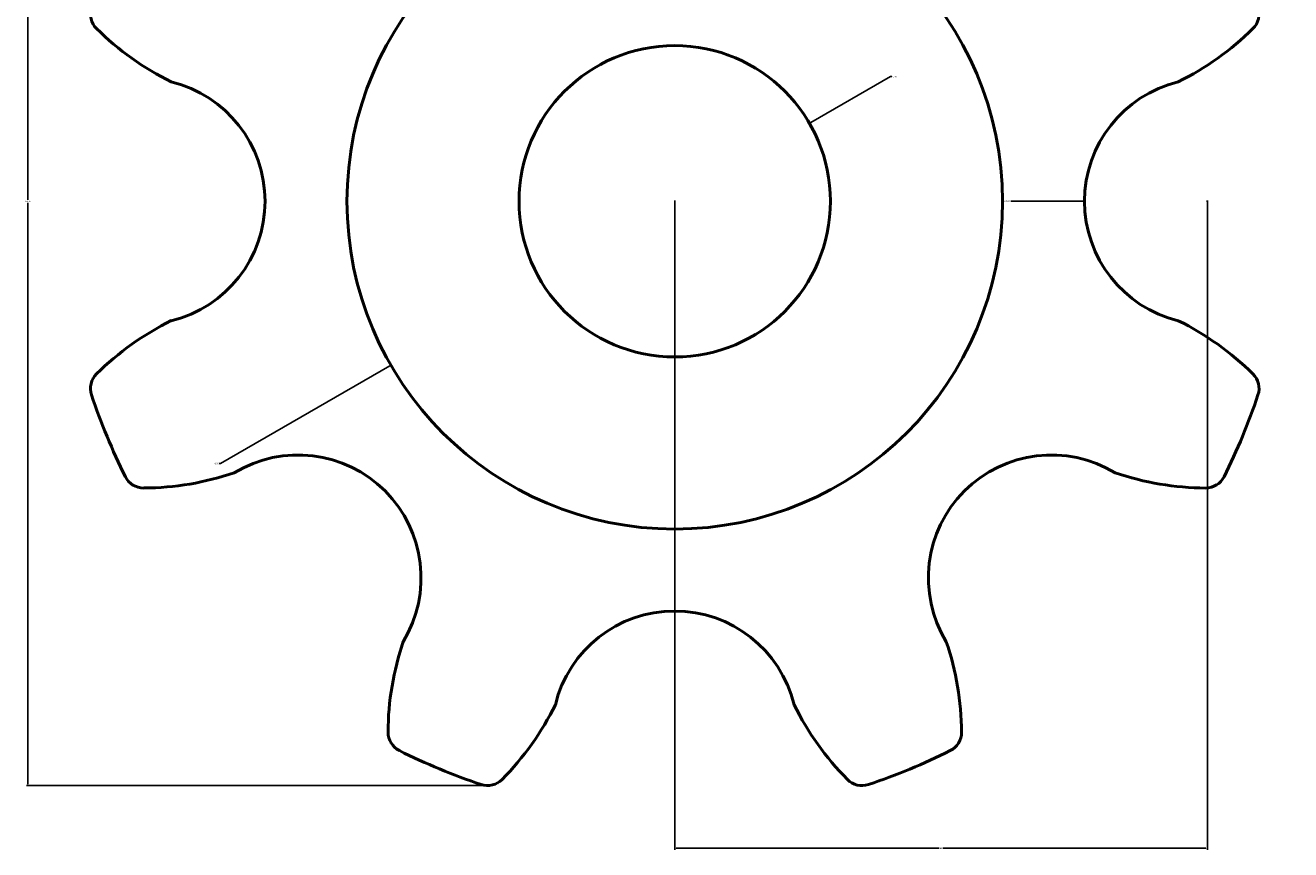
# Model space of a CAD drawing. Units: millimetres. Extents: x 7298 to 7452, y 8725 to 8883.
# Tile 1 of 2: x 7298 to 7452, y 8725 to 8826. Entities that reach past the tile are written whole.
import ezdxf

# ---------------------------------------------------------------- set-up
doc = ezdxf.new("R2010")
doc.units = ezdxf.units.MM
doc.layers.add('M-DIMS', color=2, linetype='Continuous', lineweight=18)
doc.layers.add('M-OUTL', color=7, linetype='Continuous', lineweight=50)
doc.styles.get("Standard").update_dxf_attribs({"font": 'arial.ttf'})
doc.dimstyles.get("Standard").update_dxf_attribs({"dimtxt": 0.18, "dimasz": 0.18, "dimexe": 0.18, "dimexo": 0.0625, "dimgap": 0.09, "dimtad": 0, "dimtih": 1, "dimtoh": 1, "dimdec": 4, "dimzin": 0, "dimdsep": 46, "dimtxsty": 'Standard', "dimcen": 0.09, "dimadec": 0, "dimazin": 0, "dimtfac": 1, "dimtdec": 4, "dimtofl": 0, "dimtmove": 0, "dimatfit": 3, "dimfxl": 1, "dimtolj": 1, "dimtzin": 0, "dimarcsym": 0})

# ---------------------------------------------------------------- blocks, each defined once
blk = doc.blocks.new('*U1')
for centre, radius, start, end in [((-2.28, 7.71), 2.5, 89.661, 153.3674), ((-2.47, -24.79), 35, 71.2539, 89.661), ((62.53, -24.79), 75, 153.3674, 161.6326), ((-6.28, -1.94), 2.5, 161.6326, 225.339), ((16.57, 21.18), 35, 225.339, 243.7461)]:
    blk.add_arc(centre, radius, start, end)
blk = doc.blocks.new('*U2')
at = {"layer": 'M-OUTL', "color": 0, "linetype": 'ByBlock', "lineweight": -2, "transparency": 16777216}
for p, rotation in [((7350.2, 8866.09), 315.0000000000001), ((7401.68, 8866.87), 270), ((7438.63, 8831.03), 225), ((7315.15, 8777.66), 44.99999999999996), ((7439.42, 8779.56), 180), ((7403.58, 8742.6), 134.9999999999999), ((7352.11, 8741.82), 90)]:
    blk.add_blockref('*U1', p, dxfattribs=dict(at, rotation=rotation))
blk.add_blockref('*U1', (7314.36, 8829.13), dxfattribs=at)
blk = doc.blocks.new('*D4')
at = {"layer": 'Defpoints', "color": 0, "transparency": 16777216}
for p in [(7297.94, 8875.65), (7353.95, 8875.65), (7353.95, 8733.04)]:
    blk.add_point(p, dxfattribs=at)
at = {"layer": 'M-DIMS', "color": 0, "lineweight": -2, "transparency": 16777216}
for p, q in [((7353.88, 8875.65), (7297.76, 8875.65)), ((7297.94, 8875.47), (7297.94, 8804.53)), ((7297.94, 8733.22), (7297.94, 8804.16)), ((7353.88, 8733.04), (7297.76, 8733.04))]:
    blk.add_line(p, q, dxfattribs=at)
at = {"layer": 'M-DIMS', "color": 0, "transparency": 16777216}
for points in [[(7297.91, 8875.47), (7297.97, 8875.47), (7297.94, 8875.65)], [(7297.91, 8733.22), (7297.97, 8733.22), (7297.94, 8733.04)]]:
    blk.add_solid(points, dxfattribs=at)
at = {"layer": 'M-DIMS', "color": 0, "transparency": 16777216, "insert": (7297.94, 8804.34), "char_height": 0.18, "attachment_point": 5}
blk.add_mtext('\\A1;142.6', dxfattribs=at)
blk = doc.blocks.new('*D5')
at = {"layer": 'Defpoints', "color": 0, "transparency": 16777216}
for p in [(7376.89, 8804.34), (7441.89, 8804.34), (7441.89, 8725.39)]:
    blk.add_point(p, dxfattribs=at)
at = {"layer": 'M-DIMS', "color": 0, "lineweight": -2, "transparency": 16777216}
for p, q in [((7376.89, 8804.28), (7376.89, 8725.21)), ((7441.89, 8804.28), (7441.89, 8725.21)), ((7377.07, 8725.39), (7409.17, 8725.39)), ((7441.71, 8725.39), (7409.61, 8725.39))]:
    blk.add_line(p, q, dxfattribs=at)
at = {"layer": 'M-DIMS', "color": 0, "transparency": 16777216}
for points in [[(7377.07, 8725.42), (7377.07, 8725.36), (7376.89, 8725.39)], [(7441.71, 8725.42), (7441.71, 8725.36), (7441.89, 8725.39)]]:
    blk.add_solid(points, dxfattribs=at)
at = {"layer": 'M-DIMS', "color": 0, "transparency": 16777216, "insert": (7409.39, 8725.39), "char_height": 0.18, "attachment_point": 5}
blk.add_mtext('\\A1;65', dxfattribs=at)
blk = doc.blocks.new('*D6')
at = {"layer": 'Defpoints', "color": 0, "transparency": 16777216}
for p in [(7393.35, 8813.85), (7360.44, 8794.84)]:
    blk.add_point(p, dxfattribs=at)
at = {"layer": 'M-DIMS', "color": 0, "lineweight": -2, "transparency": 16777216}
for p, q in [((7403.22, 8819.55), (7393.5, 8813.94)), ((7403.4, 8819.55), (7403.22, 8819.55)), ((7376.8, 8804.34), (7376.98, 8804.34)), ((7376.89, 8804.25), (7376.89, 8804.43))]:
    blk.add_line(p, q, dxfattribs=at)
at = {"layer": 'M-DIMS', "color": 0, "transparency": 16777216}
blk.add_solid([(7393.49, 8813.96), (7393.52, 8813.91), (7393.35, 8813.85)], dxfattribs=at)
at = {"layer": 'M-DIMS', "color": 0, "transparency": 16777216, "insert": (7403.72, 8819.55), "char_height": 0.18, "attachment_point": 5}
blk.add_mtext('\\A1;∅38', dxfattribs=at)
blk = doc.blocks.new('*D7')
at = {"layer": 'Defpoints', "color": 0, "transparency": 16777216}
for p in [(7411.53, 8824.34), (7342.25, 8784.34)]:
    blk.add_point(p, dxfattribs=at)
at = {"layer": 'M-DIMS', "color": 0, "lineweight": -2, "transparency": 16777216}
for p, q in [((7376.8, 8804.34), (7376.98, 8804.34)), ((7376.89, 8804.25), (7376.89, 8804.43)), ((7321.47, 8772.34), (7342.1, 8784.25)), ((7321.29, 8772.34), (7321.47, 8772.34))]:
    blk.add_line(p, q, dxfattribs=at)
at = {"layer": 'M-DIMS', "color": 0, "transparency": 16777216}
blk.add_solid([(7342.08, 8784.28), (7342.11, 8784.23), (7342.25, 8784.34)], dxfattribs=at)
at = {"layer": 'M-DIMS', "color": 0, "transparency": 16777216, "insert": (7320.97, 8772.34), "char_height": 0.18, "attachment_point": 5}
blk.add_mtext('\\A1;∅80', dxfattribs=at)
blk = doc.blocks.new('*D8')
at = {"layer": 'Defpoints', "color": 0, "transparency": 16777216}
for p in [(7426.89, 8804.35), (7441.89, 8804.34)]:
    blk.add_point(p, dxfattribs=at)
at = {"layer": 'M-DIMS', "color": 0, "lineweight": -2, "transparency": 16777216}
for p, q in [((7417.89, 8804.35), (7426.71, 8804.35)), ((7441.8, 8804.34), (7441.98, 8804.34)), ((7441.89, 8804.25), (7441.89, 8804.43))]:
    blk.add_line(p, q, dxfattribs=at)
at = {"layer": 'M-DIMS', "color": 0, "transparency": 16777216}
blk.add_solid([(7426.71, 8804.38), (7426.71, 8804.32), (7426.89, 8804.35)], dxfattribs=at)
at = {"layer": 'M-DIMS', "color": 0, "transparency": 16777216, "insert": (7417.39, 8804.35), "char_height": 0.18, "attachment_point": 5}
blk.add_mtext('\\A1;8X R15', dxfattribs=at)

msp = doc.modelspace()

# ---------------------------------------------------------------- linework, layer by layer
at = {"layer": 'M-OUTL'}
for radius in [40, 19]:
    msp.add_circle((7376.89, 8804.34), radius, dxfattribs=at)
for centre, start, end in [((7311.89, 8804.34), 283.7128, 76.2872), ((7441.89, 8804.34), 103.7128, 256.2872), ((7330.93, 8758.38), 328.7128, 121.2872), ((7422.85, 8758.38), 58.7128, 211.2872), ((7376.89, 8739.34), 13.7128, 166.2872)]:
    msp.add_arc(centre, 15, start, end, dxfattribs=at)

# ---------------------------------------------------------------- block references
msp.add_blockref('*U2', (0, 0), dxfattribs=at)

# ---------------------------------------------------------------- dimensions: what is measured, and where the dimension line sits
at = {"layer": 'M-DIMS'}
dim = msp.add_linear_dim(base=(7297.94, 8875.65), p1=(7353.95, 8733.04), p2=(7353.95, 8875.65), angle=90, dimstyle='Standard', override={"dimdec": 1, "dimlfac": 1, "dimrnd": 0, "dimzin": 0, "dimdsep": 46, "dimlunit": 2}, dxfattribs=at)
dim.commit()
dim.dimension.update_dxf_attribs({"geometry": '*D4', "text_midpoint": (7297.94, 8804.34)})
for p1, p2, picture, middle in [((7411.53, 8824.34), (7342.25, 8784.34), '*D7', (7320.97, 8772.34)), ((7360.44, 8794.84), (7393.35, 8813.85), '*D6', (7403.72, 8819.55))]:
    dim = msp.add_diameter_dim_2p(p1=p1, p2=p2, dimstyle='Standard', override={"dimdec": 0, "dimlfac": 1, "dimrnd": 0, "dimzin": 0, "dimdsep": 46, "dimlunit": 2}, dxfattribs=at)
    dim.commit()
    dim.dimension.update_dxf_attribs({"geometry": picture, "text_midpoint": middle, "dimtype": 163})
dim = msp.add_linear_dim(base=(7441.89, 8725.39), p1=(7376.89, 8804.34), p2=(7441.89, 8804.34), dimstyle='Standard', override={"dimdec": 0, "dimlfac": 1, "dimrnd": 0, "dimzin": 0, "dimdsep": 46, "dimlunit": 2}, dxfattribs=at)
dim.commit()
dim.dimension.update_dxf_attribs({"geometry": '*D5', "text_midpoint": (7409.39, 8725.39)})
dim = msp.add_radius_dim(center=(7441.89, 8804.34), mpoint=(7426.89, 8804.35), text='8X <>', dimstyle='Standard', override={"dimdec": 0, "dimlfac": 1, "dimrnd": 0, "dimzin": 0, "dimdsep": 46, "dimlunit": 2}, dxfattribs=at)
dim.commit()
dim.dimension.update_dxf_attribs({"geometry": '*D8', "text_midpoint": (7417.89, 8804.35), "dimtype": 164})

doc.saveas('drawing.dxf')
